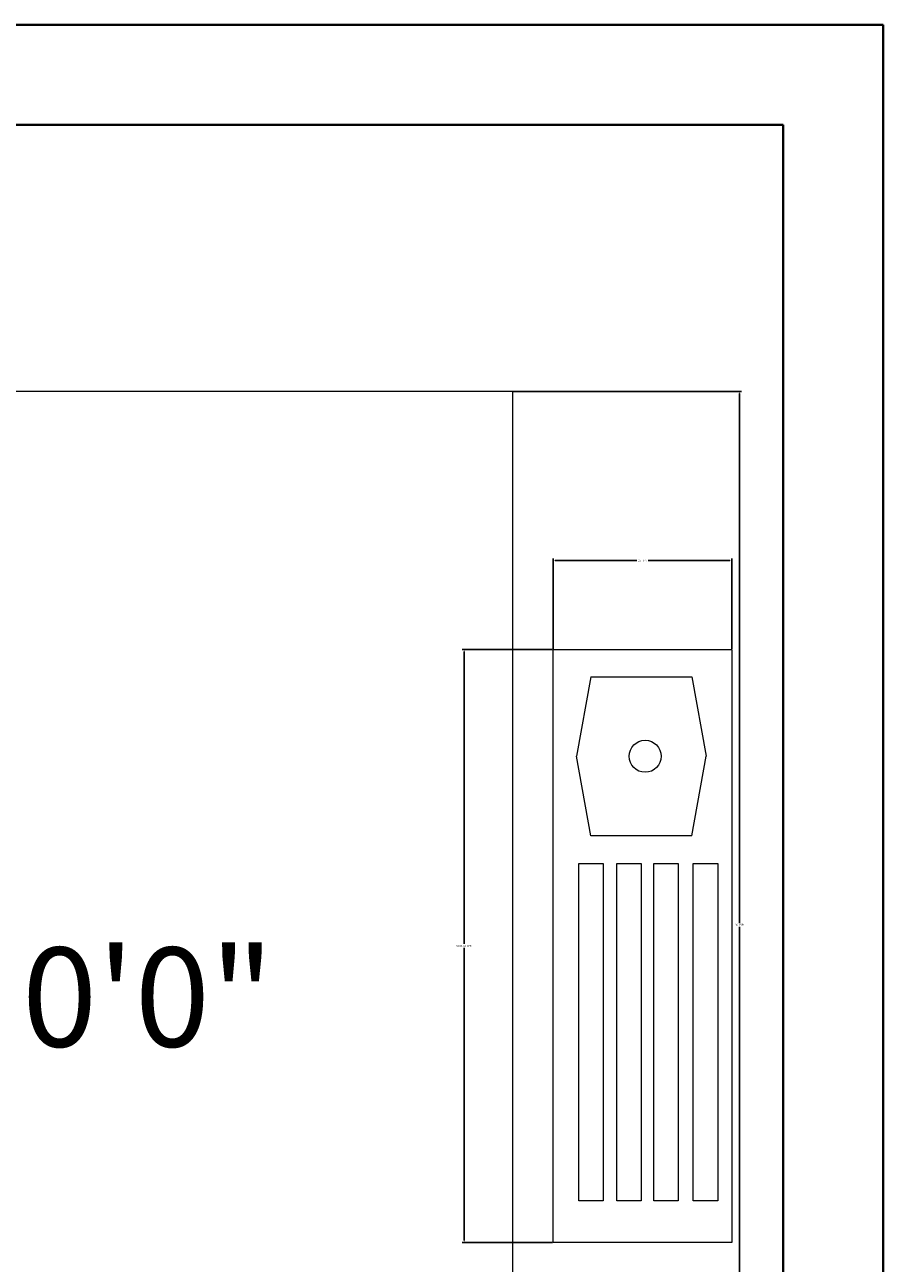
# Model space of a CAD drawing. Units: inches. Extents: x -46 to 1145, y -527 to 760.
# Tile 52 of 57: x 432 to 509, y 548 to 660. Entities that reach past the tile are written whole.
import ezdxf

# ---------------------------------------------------------------- set-up
doc = ezdxf.new("R2010")
doc.units = ezdxf.units.IN
doc.header["$MEASUREMENT"] = 0
for name, color, linetype, lineweight in [('A-ANNO-DIMS', 2, 'Continuous', 18), ('A-AREA-IDEN', 1, 'Continuous', 18), ('A-FLOR-CASE', 32, 'Continuous', 18), ('A-FLOR-FIXT', 9, 'Continuous', 18), ('WALLS', 4, 'Continuous', 40)]:
    doc.layers.add(name, color=color, linetype=linetype, lineweight=lineweight)
doc.styles.get("Standard").update_dxf_attribs({"font": 'arial.ttf'})
doc.dimstyles.get("Standard").update_dxf_attribs({"dimtxt": 0.18, "dimasz": 0.18, "dimexe": 0.18, "dimexo": 0.0625, "dimgap": 0.09, "dimtad": 0, "dimtih": 1, "dimtoh": 1, "dimdec": 0, "dimzin": 0, "dimdsep": 46, "dimlunit": 3, "dimtxsty": 'Standard', "dimcen": 0.09, "dimadec": 0, "dimazin": 0, "dimtfac": 1, "dimtdec": 0, "dimtofl": 0, "dimtmove": 0, "dimatfit": 3, "dimfxl": 1, "dimtolj": 1, "dimtzin": 0, "dimarcsym": 0})

# ---------------------------------------------------------------- blocks, each defined once
blk = doc.blocks.new('SINK-DRAINBOARD')
for p, q in [((3.38, 50.9), (2.09, 43.74)), ((12.47, 50.9), (13.77, 43.74)), ((3.38, 36.58), (2.09, 43.74)), ((12.47, 36.58), (13.77, 43.74))]:
    blk.add_line(p, q)
for points in [[(16.07, 0), (0, 0), (0, 53.35), (16.07, 53.35)], [(4.51, 3.73), (2.3, 3.73), (2.3, 34.08), (4.51, 34.08)], [(7.92, 3.73), (5.72, 3.73), (5.72, 34.08), (7.92, 34.08)], [(11.26, 3.73), (9.05, 3.73), (9.05, 34.08), (11.26, 34.08)], [(14.8, 3.73), (12.59, 3.73), (12.59, 34.08), (14.8, 34.08)]]:
    blk.add_lwpolyline(points, close=True)
for points in [[(3.38, 50.9), (12.47, 50.9)], [(12.47, 36.58), (3.38, 36.58)]]:
    blk.add_lwpolyline(points)
blk.add_circle((8.28, 43.74), 1.44)
blk = doc.blocks.new('KITCHEN-COUNTER-L')
for p, q in [((136.17, 96), (0, 96)), ((136.17, 24), (136.17, 96)), ((136.17, 0), (136.17, 24))]:
    blk.add_line(p, q)
blk = doc.blocks.new('*D680')
at = {"layer": 'A-ANNO-DIMS', "color": 0, "lineweight": -2, "transparency": 16777216}
for p, q in [((479.31, 603.3), (471.19, 603.3)), ((471.37, 603.12), (471.37, 576.8)), ((471.37, 550.12), (471.37, 576.44)), ((479.31, 549.94), (471.19, 549.94))]:
    blk.add_line(p, q, dxfattribs=at)
at = {"layer": 'A-ANNO-DIMS', "color": 0, "transparency": 16777216}
for points in [[(471.34, 603.12), (471.4, 603.12), (471.37, 603.3)], [(471.34, 550.12), (471.4, 550.12), (471.37, 549.94)]]:
    blk.add_solid(points, dxfattribs=at)
at = {"layer": 'Defpoints', "color": 0, "transparency": 16777216}
for p in [(471.37, 603.3), (479.37, 603.3), (479.37, 549.94)]:
    blk.add_point(p, dxfattribs=at)
at = {"layer": 'A-ANNO-DIMS', "color": 0, "transparency": 16777216, "insert": (471.37, 576.62), "char_height": 0.18, "attachment_point": 5}
blk.add_mtext('\\A1;SINK 53 TYP.', dxfattribs=at)
blk = doc.blocks.new('*D681')
at = {"layer": 'A-ANNO-DIMS', "color": 0, "lineweight": -2, "transparency": 16777216}
for p, q in [((479.37, 603.36), (479.37, 611.48)), ((479.55, 611.3), (486.89, 611.3)), ((495.26, 611.3), (487.93, 611.3)), ((495.44, 603.36), (495.44, 611.48))]:
    blk.add_line(p, q, dxfattribs=at)
at = {"layer": 'A-ANNO-DIMS', "color": 0, "transparency": 16777216}
for points in [[(479.55, 611.33), (479.55, 611.27), (479.37, 611.3)], [(495.26, 611.33), (495.26, 611.27), (495.44, 611.3)]]:
    blk.add_solid(points, dxfattribs=at)
at = {"layer": 'Defpoints', "color": 0, "transparency": 16777216}
for p in [(495.44, 611.3), (479.37, 603.3), (495.44, 603.3)]:
    blk.add_point(p, dxfattribs=at)
at = {"layer": 'A-ANNO-DIMS', "color": 0, "transparency": 16777216, "insert": (487.41, 611.3), "char_height": 0.18, "attachment_point": 5}
blk.add_mtext('\\A1;16 TYP.', dxfattribs=at)
blk = doc.blocks.new('*D683')
at = {"layer": 'A-ANNO-DIMS', "color": 0, "lineweight": -2, "transparency": 16777216}
for p, q in [((475.79, 626.52), (496.33, 626.52)), ((496.15, 626.34), (496.15, 578.7)), ((496.15, 530.7), (496.15, 578.34)), ((475.79, 530.52), (496.33, 530.52))]:
    blk.add_line(p, q, dxfattribs=at)
at = {"layer": 'A-ANNO-DIMS', "color": 0, "transparency": 16777216}
for points in [[(496.12, 626.34), (496.18, 626.34), (496.15, 626.52)], [(496.12, 530.7), (496.18, 530.7), (496.15, 530.52)]]:
    blk.add_solid(points, dxfattribs=at)
at = {"layer": 'Defpoints', "color": 0, "transparency": 16777216}
for p in [(475.73, 626.52), (496.15, 626.52), (475.73, 530.52)]:
    blk.add_point(p, dxfattribs=at)
at = {"layer": 'A-ANNO-DIMS', "color": 0, "transparency": 16777216, "insert": (496.15, 578.52), "char_height": 0.18, "attachment_point": 5}
blk.add_mtext('\\A1;96 TYP.', dxfattribs=at)

msp = doc.modelspace()

# ---------------------------------------------------------------- linework, layer by layer
at = {"layer": 'WALLS'}
for p, q in [((339.5637, 659.5176), (509.0637, 659.5176)), ((509.0637, 659.5176), (509.0637, 221.5176)), ((339.5637, 650.5176), (500.0637, 650.5176)), ((500.0637, 650.5176), (500.0637, 524.5176))]:
    msp.add_line(p, q, dxfattribs=at)

# ---------------------------------------------------------------- block references
at = {"layer": 'A-FLOR-CASE'}
msp.add_blockref('KITCHEN-COUNTER-L', (339.564, 530.518), dxfattribs=at)
at = {"layer": 'A-FLOR-FIXT'}
msp.add_blockref('SINK-DRAINBOARD', (479.373, 549.944), dxfattribs=at)

# ---------------------------------------------------------------- texts
at = {"layer": 'A-AREA-IDEN'}
msp.add_text('13\'4.5" X 10\'0"', height=8.923264, dxfattribs=at).set_placement((372.8531, 567.5501))

# ---------------------------------------------------------------- dimensions: what is measured, and where the dimension line sits
at = {"layer": 'A-ANNO-DIMS'}
for base, p1, p2, text, picture, middle in [((496.1541, 626.5176), (475.7292, 530.5176), (475.7292, 626.5176), '<> TYP.', '*D683', (496.1541, 578.5176)), ((471.3706, 603.2962), (479.3735, 549.944), (479.3735, 603.2962), 'SINK <> TYP.', '*D680', (471.3706, 576.6201))]:
    dim = msp.add_linear_dim(base=base, p1=p1, p2=p2, angle=90, text=text, dimstyle='Standard', override={"dimdec": 0, "dimlfac": 1, "dimrnd": 0, "dimzin": 0, "dimdsep": 46, "dimlunit": 2}, dxfattribs=at)
    dim.commit()
    dim.dimension.update_dxf_attribs({"geometry": picture, "text_midpoint": middle})
dim = msp.add_linear_dim(base=(495.4406, 611.299), p1=(479.3735, 603.2962), p2=(495.4406, 603.2962), text='<> TYP.', dimstyle='Standard', override={"dimdec": 0, "dimlfac": 1, "dimrnd": 0, "dimzin": 0, "dimdsep": 46, "dimlunit": 2}, dxfattribs=at)
dim.commit()
dim.dimension.update_dxf_attribs({"geometry": '*D681', "text_midpoint": (487.407, 611.299)})

doc.saveas('drawing.dxf')
